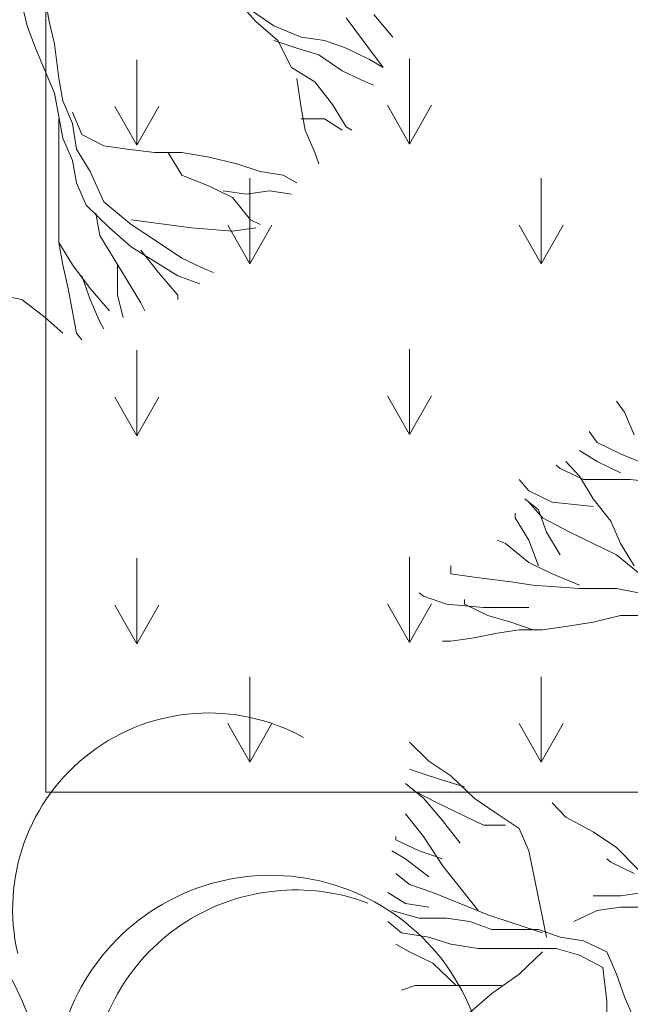
# Model space of a CAD drawing. Units: millimetres. Extents: x 595116 to 630915, y 909473 to 920225.
# Tile 16 of 134: x 629534 to 629559, y 919176 to 919216. Entities that reach past the tile are written whole.
import ezdxf

# ---------------------------------------------------------------- set-up
doc = ezdxf.new("R2010")
doc.units = ezdxf.units.MM
doc.layers.add('Dimension', color=3, linetype='Continuous', lineweight=18)
doc.layers.add('L-PLNT', color=85, linetype='Continuous', lineweight=13)
doc.styles.get("Standard").update_dxf_attribs({"font": 'arial.ttf'})
doc.dimstyles.new('ISO-25', dxfattribs={"dimtxt": 9, "dimasz": 6, "dimexe": 1.25, "dimexo": 0.625, "dimtad": 1, "dimlunit": 4, "dimtxsty": 'Standard', "dimcen": 2.5, "dimadec": 0, "dimazin": 0, "dimtfac": 1, "dimtmove": 0, "dimatfit": 3, "dimfxl": 1, "dimarcsym": 0})

# ---------------------------------------------------------------- blocks, each defined once
blk = doc.blocks.new('tree')
for centre, radius, start, end in [((629595.141, 919296.95), 5.184, 352.032, 57.0714), ((629604.232, 919296.737), 3.791, 61.1347, 193.108), ((629569.835, 919289.496), 31.168, 13.149, 20.5076), ((629594.259, 919292.132), 6.965, 7.4001, 94.0059), ((629589.446, 919288.922), 12.167, 24.2477, 54.3726), ((629605.429, 919293.205), 4.185, 348.9977, 176.315), ((629605.915, 919293.144), 3.963, 69.3845, 175.231), ((629595.377, 919292.044), 4.722, 54.2484, 144.2167), ((629594.88, 919291.171), 5.506, 43.8672, 89.4805), ((629597.025, 919289.989), 5.01, 36.0581, 170.6542), ((629603.809, 919290.469), 3.92, 343.886, 112.2662), ((629596.464, 919289.874), 4.4, 52.9074, 159.3471), ((629598.153, 919288.998), 5.103, 105.3576, 208.8973), ((629597.068, 919289.758), 3.768, 80.4816, 161.0664), ((629601.247, 919287.941), 5.545, 101.0419, 191.8692), ((629614.329, 919289.554), 13.748, 164.5925, 192.323), ((629600.849, 919288.894), 4.324, 322.5461, 85.805), ((629602.329, 919287.957), 5.355, 355.2141, 94.8217), ((629602.391, 919286.088), 6.769, 99.681, 184.5451), ((629600.275, 919288.191), 4.585, 338.7925, 77.6921), ((629626.813, 919287.645), 25.579, 169.0753, 185.2889)]:
    blk.add_arc(centre, radius, start, end)
blk = doc.blocks.new('A$C143125F4')
for p, q in [((0.9464, 4.341), (0.9136, 4.3858)), ((0.9847, 4.2514), (0.9464, 4.341)), ((0.837, 4.22), (0.8042, 4.2648)), ((0.93, 4.1752), (0.837, 4.22)), ((0.837, 4.1439), (0.7659, 4.1887)), ((1.0394, 4.1304), (0.93, 4.1752)), ((0.6893, 4.117), (0.6729, 4.1304)), ((0.7659, 4.0856), (0.7112, 4.1439)), ((0.93, 4.0991), (0.837, 4.1439)), ((0.7823, 4.0722), (0.6893, 4.117)), ((0.5635, 4.0274), (0.5252, 4.0722)), ((0.8206, 3.996), (0.7659, 4.0856)), ((0.9683, 4.0722), (0.7823, 4.0722)), ((1.1488, 4.0543), (0.9683, 4.0722)), ((0.6565, 3.9826), (0.5635, 4.0274)), ((0.6018, 3.9512), (0.5471, 3.996)), ((0.6182, 3.9199), (0.5635, 3.9826)), ((0.8206, 3.9647), (0.6565, 3.9826)), ((0.8917, 3.9064), (0.8206, 3.996)), ((0.5088, 3.9199), (0.5088, 3.9378)), ((0.6346, 3.8616), (0.6018, 3.9512)), ((0.5635, 3.8303), (0.5088, 3.9199)), ((0.7276, 3.8616), (0.6182, 3.9199)), ((0.93, 3.8168), (0.8917, 3.9064)), ((0.6893, 3.772), (0.6346, 3.8616)), ((0.9136, 3.772), (0.7276, 3.8616)), ((0.4705, 3.8168), (0.4376, 3.8303)), ((0.5635, 3.7407), (0.4705, 3.8168)), ((0.6018, 3.7272), (0.5635, 3.8303)), ((0.9847, 3.7272), (0.93, 3.8168)), ((0.6565, 3.6959), (0.5635, 3.7407)), ((1.023, 3.6824), (0.9136, 3.772)), ((0.2516, 3.6959), (0.2516, 3.7272)), ((0.3446, 3.6824), (0.2516, 3.6959)), ((0.4923, 3.6645), (0.3446, 3.6824)), ((0.5799, 3.6511), (0.4923, 3.6645)), ((0.7659, 3.6511), (0.6565, 3.6959)), ((0.1422, 3.6063), (0.1258, 3.6197)), ((0.7659, 3.6376), (0.5799, 3.6511)), ((0.9136, 3.6376), (0.7659, 3.6376)), ((1.0011, 3.6197), (0.9136, 3.6376)), ((0.2352, 3.5749), (0.1422, 3.6063)), ((0.3063, 3.5749), (0.3063, 3.5928)), ((0.3829, 3.5615), (0.2352, 3.5749)), ((0.3993, 3.5301), (0.3063, 3.5749)), ((0.5635, 3.5615), (0.3829, 3.5615)), ((0.4923, 3.5032), (0.3993, 3.5301)), ((0.5799, 3.4719), (0.4923, 3.5032)), ((0.8206, 3.5032), (0.7112, 3.4853)), ((0.93, 3.5301), (0.8206, 3.5032)), ((1.0777, 3.5301), (0.93, 3.5301)), ((0.5252, 3.4719), (0.4376, 3.4584)), ((0.6182, 3.4719), (0.5252, 3.4719)), ((0.7112, 3.4853), (0.6182, 3.4719)), ((0.2516, 3.4271), (0.2188, 3.4271)), ((0.3446, 3.4405), (0.2516, 3.4271)), ((0.4376, 3.4584), (0.3446, 3.4405)), ((0.1641, 2.9477), (0.0875, 3.0239)), ((0.1258, 2.9029), (0.0875, 2.9164)), ((0.2516, 2.8895), (0.1641, 2.9477)), ((0.2188, 2.8716), (0.1258, 2.9029)), ((0.3063, 2.8447), (0.2188, 2.8716)), ((0.3446, 2.7999), (0.2516, 2.8895)), ((0.1422, 2.7999), (0.0711, 2.8581)), ((0.1094, 2.8268), (0.0711, 2.8581)), ((0.1969, 2.782), (0.1094, 2.8268)), ((0.2188, 2.7103), (0.1422, 2.7999)), ((0.4376, 2.7372), (0.3446, 2.7999)), ((0.3829, 2.6924), (0.1969, 2.782)), ((0.7112, 2.7238), (0.6565, 2.782)), ((0.1422, 2.6476), (0.0711, 2.7372)), ((0.5252, 2.679), (0.4376, 2.7372)), ((0.8206, 2.6655), (0.7112, 2.7238)), ((0.2899, 2.6207), (0.2188, 2.7103)), ((0.4705, 2.6924), (0.3829, 2.6924)), ((0.5635, 2.5894), (0.5252, 2.679)), ((0.0328, 2.6342), (0.0328, 2.6476)), ((0.2188, 2.5311), (0.1422, 2.6476)), ((0.9136, 2.6028), (0.8206, 2.6655)), ((0.1258, 2.5894), (0.0328, 2.6342)), ((1.0011, 2.5132), (0.9136, 2.6028)), ((0.0711, 2.558), (0.0164, 2.5894)), ((0.1641, 2.4863), (0.0711, 2.558)), ((0.2188, 2.558), (0.1258, 2.5894)), ((0.6346, 2.2444), (0.5635, 2.5894)), ((0.8917, 2.5446), (0.8753, 2.558)), ((0.3611, 2.3519), (0.2188, 2.5311)), ((0.9847, 2.4998), (0.8917, 2.5446)), ((0.0875, 2.455), (0.0328, 2.4998)), ((0.1805, 2.4236), (0.0875, 2.455)), ((0.0711, 2.3788), (0, 2.4236)), ((0.3993, 2.334), (0.1805, 2.4236)), ((0.93, 2.4102), (0.8206, 2.4102)), ((1.023, 2.4236), (0.93, 2.4102)), ((0.1641, 2.3654), (0.0711, 2.3788)), ((0.93, 2.3654), (0.837, 2.3519)), ((1.2965, 2.3654), (0.93, 2.3654)), ((0.0164, 2.3519), (0.1258, 2.3206)), ((0.1258, 2.3206), (0.2352, 2.3206)), ((0.2352, 2.3206), (0.3282, 2.3071)), ((0.6182, 2.2623), (0.3993, 2.334)), ((0.837, 2.3519), (0.744, 2.3071)), ((0.0547, 2.2623), (0, 2.3071)), ((0.3282, 2.3071), (0.4158, 2.2758)), ((0.1641, 2.2444), (0.0547, 2.2623)), ((0.2516, 2.2175), (0.1641, 2.2444)), ((0.4158, 2.2758), (0.6018, 2.2758)), ((0.6018, 2.2758), (0.6893, 2.2444)), ((0.6893, 2.2444), (0.7823, 2.231)), ((0.0875, 2.1862), (0.0328, 2.2175)), ((0.3611, 2.1996), (0.2516, 2.2175)), ((0.7823, 2.231), (0.8753, 2.1862)), ((0.1805, 2.1414), (0.0875, 2.1862)), ((0.6729, 2.1996), (0.3611, 2.1996)), ((0.6182, 2.1862), (0.5252, 2.0966)), ((0.7659, 2.1727), (0.6729, 2.1996)), ((0.8589, 2.1235), (0.7659, 2.1727)), ((0.8753, 2.1862), (0.9136, 2.0966)), ((0.2735, 2.0518), (0.1805, 2.1414)), ((0.8753, 1.9891), (0.8589, 2.1235)), ((0.5252, 2.0966), (0.4158, 2.0204)), ((0.9136, 2.0966), (0.9464, 2.007)), ((0.1094, 2.0518), (0.0547, 2.0339)), ((0.4541, 2.0518), (0.1094, 2.0518)), ((0.4158, 2.0204), (0.3282, 1.9443)), ((0.9464, 2.007), (0.9847, 1.9174)), ((0.8753, 1.8412), (0.8753, 1.9891)), ((3.1237, 1.4515), (3.1018, 1.5411)), ((3.1948, 1.559), (3.2112, 1.4694)), ((3.9442, 1.5724), (4.0372, 1.4694)), ((3.999, 1.5276), (4.1084, 1.4515)), ((4.5077, 1.4963), (4.5843, 1.4067)), ((3.2112, 1.4694), (3.2331, 1.3798)), ((4.0372, 1.4694), (4.1248, 1.3932)), ((4.3983, 1.4828), (4.4749, 1.3798)), ((3.1565, 1.3619), (3.1237, 1.4515)), ((4.1084, 1.4515), (4.2178, 1.4067)), ((3.2331, 1.3798), (3.2495, 1.2409)), ((4.1084, 1.3932), (4.2014, 1.3619)), ((4.1248, 1.3932), (4.1795, 1.2857)), ((4.2178, 1.4067), (4.3108, 1.3932)), ((4.3108, 1.3932), (4.3983, 1.3619)), ((4.4749, 1.3798), (4.546, 1.2857)), ((3.2331, 1.1827), (3.1565, 1.3619)), ((4.2014, 1.3619), (4.2889, 1.335)), ((4.3983, 1.3619), (4.4913, 1.3171)), ((4.2889, 1.335), (4.3819, 1.2723)), ((4.4913, 1.3171), (4.546, 1.2857)), ((4.1795, 1.2857), (4.2725, 1.2275)), ((4.3819, 1.2723), (4.4749, 1.2275)), ((3.2495, 1.2409), (3.2659, 1.1513)), ((4.2014, 1.2409), (4.2178, 1.1244)), ((4.2725, 1.2275), (4.3436, 1.1379)), ((4.4749, 1.2275), (4.5077, 1.214)), ((3.2659, 1.0035), (3.2331, 1.1827)), ((3.2659, 1.1513), (3.3042, 1.0617)), ((3.3042, 1.1065), (3.3425, 1.0169)), ((4.2178, 1.1244), (4.2342, 1.0348)), ((4.3436, 1.1379), (4.3983, 1.0483)), ((3.2495, 1.0796), (3.2495, 0.5869)), ((3.3042, 1.0617), (3.3206, 0.9587)), ((4.2178, 1.0796), (4.3108, 1.0796)), ((4.3108, 1.0796), (4.3819, 1.0348)), ((4.2342, 1.0348), (4.2725, 0.9452)), ((4.3983, 1.0483), (4.4202, 1.0348)), ((3.3042, 0.9139), (3.2659, 1.0035)), ((3.3425, 1.0169), (3.43, 0.9721)), ((3.3206, 0.9587), (3.3753, 0.8691)), ((3.43, 0.9721), (3.523, 0.9587)), ((3.523, 0.9587), (3.6324, 0.9452)), ((3.6324, 0.9452), (3.7418, 0.9452)), ((3.6871, 0.9452), (3.7418, 0.8557)), ((3.7418, 0.9452), (3.8512, 0.9273)), ((4.2725, 0.9452), (4.2889, 0.9005)), ((3.3206, 0.8243), (3.3042, 0.9139)), ((3.8512, 0.9273), (3.9607, 0.9005)), ((3.3753, 0.8691), (3.43, 0.7481)), ((3.9607, 0.9005), (4.0537, 0.8691)), ((4.0537, 0.8691), (4.1467, 0.8557)), ((3.7418, 0.8557), (3.8512, 0.8109)), ((4.1467, 0.8557), (4.2014, 0.8243)), ((3.3589, 0.7347), (3.3206, 0.8243)), ((3.8512, 0.8109), (3.9442, 0.7661)), ((3.906, 0.7929), (3.999, 0.7795)), ((3.999, 0.7795), (4.092, 0.7929)), ((4.092, 0.7929), (4.1795, 0.7795)), ((3.43, 0.7481), (3.5394, 0.6585)), ((3.9442, 0.7661), (4.0154, 0.6765)), ((3.4519, 0.6451), (3.3589, 0.7347)), ((3.3972, 0.7033), (3.4136, 0.6137)), ((3.5394, 0.6765), (3.7801, 0.6451)), ((4.0154, 0.6765), (4.0537, 0.6585)), ((3.5394, 0.5689), (3.4519, 0.6451)), ((3.5394, 0.6585), (3.6488, 0.5869)), ((3.7801, 0.6451), (3.9442, 0.6317)), ((3.9442, 0.6317), (4.0372, 0.6451)), ((3.4136, 0.6137), (3.5777, 0.3449)), ((3.2495, 0.5869), (3.3042, 0.4973)), ((3.2495, 0.5869), (3.2659, 0.4973)), ((3.7254, 0.4525), (3.5394, 0.5689)), ((3.5777, 0.5555), (3.6488, 0.4659)), ((3.6488, 0.5869), (3.7418, 0.5241)), ((3.7418, 0.5241), (3.8348, 0.4793)), ((3.2659, 0.4973), (3.2878, 0.4032)), ((3.3042, 0.4973), (3.3753, 0.4032)), ((3.4847, 0.4973), (3.4847, 0.3763)), ((3.8348, 0.4793), (3.8677, 0.4659)), ((3.3425, 0.4525), (3.3753, 0.3584)), ((3.6488, 0.4659), (3.7254, 0.3763)), ((3.813, 0.4211), (3.7254, 0.4525)), ((3.2878, 0.4032), (3.3206, 0.224)), ((3.3753, 0.4032), (3.4519, 0.3136)), ((3.0143, 0.3763), (3.1018, 0.3584)), ((3.1018, 0.3584), (3.1948, 0.2867)), ((3.3753, 0.3584), (3.4136, 0.2688)), ((3.4847, 0.3763), (3.5066, 0.2867)), ((3.7254, 0.3763), (3.7254, 0.3584)), ((3.5777, 0.3449), (3.5941, 0.3136)), ((3.1948, 0.2867), (3.2659, 0.224)), ((3.4136, 0.2688), (3.43, 0.2419)), ((3.3206, 0.224), (3.3425, 0.1971))]:
    blk.add_line(p, q)
blk = doc.blocks.new('LAWN-GRASS-TUFT')
blk.add_line((0.892, 3.485), (0.892, 0))
blk.add_lwpolyline([(0, 1.577), (0.892, 0), (1.785, 1.577)])
blk = doc.blocks.new('*D216')
at = {"layer": 'Defpoints', "color": 0, "transparency": 16777216}
for p in [(629505.041, 919411.828), (629743.541, 919411.928), (629743.541, 918832.378)]:
    blk.add_point(p, dxfattribs=at)
at = {"layer": 'Dimension', "color": 0, "lineweight": -2, "transparency": 16777216}
for p, q in [((629505.041, 919411.203), (629505.041, 918831.128)), ((629743.541, 919411.303), (629743.541, 918831.128)), ((629511.041, 918832.378), (629737.541, 918832.378))]:
    blk.add_line(p, q, dxfattribs=at)
at = {"layer": 'Dimension', "color": 0, "transparency": 16777216}
for points in [[(629511.041, 918833.378), (629511.041, 918831.378), (629505.041, 918832.378)], [(629737.541, 918833.378), (629737.541, 918831.378), (629743.541, 918832.378)]]:
    blk.add_solid(points, dxfattribs=at)
at = {"layer": 'Dimension', "color": 0, "transparency": 16777216, "insert": (629624.291, 918837.656), "char_height": 9, "attachment_point": 5}
blk.add_mtext('19\'-10 1/2"', dxfattribs=at)

msp = doc.modelspace()

# ---------------------------------------------------------------- linework, layer by layer
at = {"layer": 'L-PLNT'}
for p, q in [((629535.274, 919266.009), (629535.274, 919184.917)), ((629535.274, 919184.917), (629800.951, 919184.917))]:
    msp.add_line(p, q, dxfattribs=at)

# ---------------------------------------------------------------- block references
for name, p, xscale, yscale, zscale in [('A$C143125F4', (629502.654, 919201.332), 10.20167662382051, 10.20167662382051, 10.20167662382051), ('A$C143125F4', (629549.214, 919156.111), 10.20167662382051, 10.20167662382051, 10.20167662382051), ('tree', (-697468.256, -1018411.841), 2.107689410566463, 2.107689410566463, 2.107689410566463)]:
    msp.add_blockref(name, p, dxfattribs=dict(at, xscale=xscale, yscale=yscale, zscale=zscale))
for p in [(629538.093, 919211.275), (629549.207, 919211.325), (629542.7, 919206.447), (629554.573, 919206.447), (629538.093, 919199.437), (629549.207, 919199.487), (629538.093, 919190.967), (629549.207, 919191.017), (629542.7, 919186.14), (629554.573, 919186.14)]:
    msp.add_blockref('LAWN-GRASS-TUFT', p, dxfattribs=at)

# ---------------------------------------------------------------- dimensions: what is measured, and where the dimension line sits
at = {"layer": 'Dimension'}
dim = msp.add_linear_dim(base=(629743.541, 918832.378), p1=(629505.041, 919411.828), p2=(629743.541, 919411.928), dimstyle='ISO-25', override={"dimdec": 1, "dimlfac": 1, "dimrnd": 0, "dimzin": 1, "dimdsep": 46, "dimlunit": 4, "dimfrac": 2}, dxfattribs=at)
dim.commit()
dim.dimension.update_dxf_attribs({"geometry": '*D216', "text_midpoint": (629624.291, 918837.656)})

doc.saveas('drawing.dxf')
